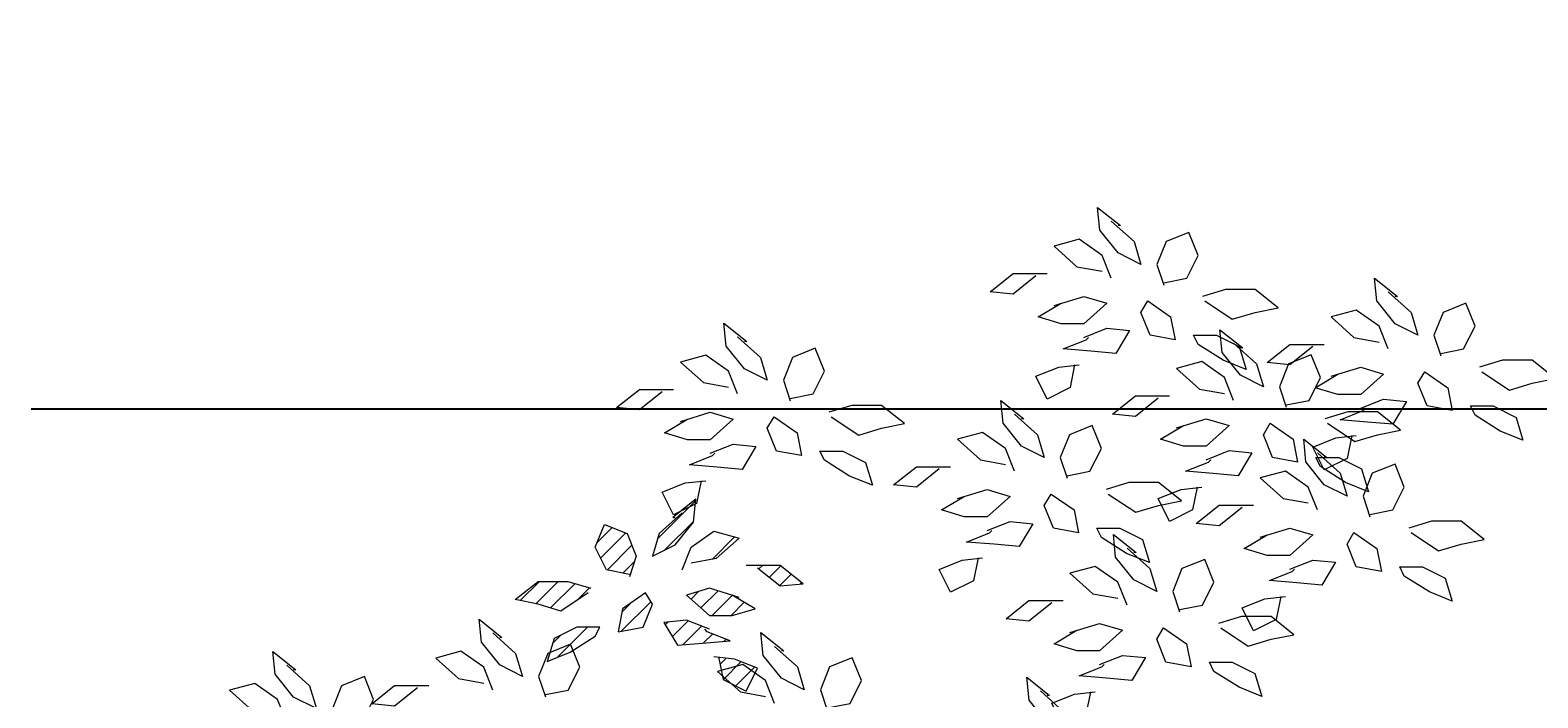
# Model space of a CAD drawing. Units: inches. Extents: x 1770 to 2988, y 1161 to 3221.
# Tile 42 of 44: x 2655 to 2745, y 2825 to 2865. Entities that reach past the tile are written whole.
import ezdxf

# ---------------------------------------------------------------- set-up
doc = ezdxf.new("R2010")
doc.units = ezdxf.units.IN
doc.layers.add('A-ANNO-DIMS', color=2, linetype='Continuous', lineweight=18)
doc.layers.add('trees1', color=250, linetype='Continuous', lineweight=13)
doc.styles.get("Standard").update_dxf_attribs({"font": 'arial.ttf'})
doc.dimstyles.get("Standard").update_dxf_attribs({"dimtxt": 0.18, "dimasz": 0.18, "dimexe": 0.18, "dimexo": 0.0625, "dimgap": 0.09, "dimtad": 0, "dimtih": 1, "dimtoh": 1, "dimdec": 4, "dimzin": 0, "dimdsep": 46, "dimtxsty": 'Standard', "dimcen": 0.09, "dimadec": 0, "dimazin": 0, "dimtfac": 1, "dimtdec": 4, "dimtofl": 0, "dimtmove": 0, "dimatfit": 3, "dimfxl": 1, "dimtolj": 1, "dimtzin": 0, "dimarcsym": 0})

# ---------------------------------------------------------------- blocks, each defined once
blk = doc.blocks.new('*X8')
at = {"color": 0}
for p, q in [((0.637, -0.8479), (0.6441, -0.8408)), ((0.6463, -0.8563), (0.6624, -0.8402)), ((0.6568, -0.8635), (0.676, -0.8443)), ((0.6745, -0.8635), (0.687, -0.8509))]:
    blk.add_line(p, q, dxfattribs=at)
blk = doc.blocks.new('*X14')
at = {"color": 0}
blk.add_line((0.6567, -0.8106), (0.6779, -0.7894), dxfattribs=at)
blk = doc.blocks.new('*X9')
at = {"color": 0}
for p, q in [((0.7007, -0.8195), (0.704, -0.8163)), ((0.7106, -0.8274), (0.7213, -0.8167)), ((0.7204, -0.8352), (0.7311, -0.8245)), ((0.7396, -0.8337), (0.7409, -0.8324))]:
    blk.add_line(p, q, dxfattribs=at)
blk = doc.blocks.new('*X7')
at = {"color": 0}
for p, q in [((0.6642, -0.9091), (0.6699, -0.9034)), ((0.6673, -0.9237), (0.6842, -0.9068)), ((0.6791, -0.9296), (0.6968, -0.9118))]:
    blk.add_line(p, q, dxfattribs=at)
blk = doc.blocks.new('*X11')
at = {"color": 0}
for p, q in [((0.5716, -0.8779), (0.5992, -0.8504)), ((0.5721, -0.8598), (0.5799, -0.852))]:
    blk.add_line(p, q, dxfattribs=at)
blk = doc.blocks.new('*X12')
at = {"color": 0}
for p, q in [((0.4764, -0.8494), (0.4945, -0.8313)), ((0.4911, -0.8524), (0.5122, -0.8313)), ((0.5049, -0.8563), (0.5279, -0.8333)), ((0.5296, -0.8493), (0.5415, -0.8374))]:
    blk.add_line(p, q, dxfattribs=at)
blk = doc.blocks.new('*X10')
at = {"color": 0}
for p, q in [((0.5118, -0.9024), (0.54, -0.8742)), ((0.5068, -0.8897), (0.5149, -0.8816))]:
    blk.add_line(p, q, dxfattribs=at)
blk = doc.blocks.new('*X6')
at = {"color": 0}
for p, q in [((0.6127, -0.8722), (0.6154, -0.8695)), ((0.6193, -0.8833), (0.6342, -0.8684)), ((0.6293, -0.8909), (0.6469, -0.8734)), ((0.6488, -0.8892), (0.6573, -0.8806)), ((0.6681, -0.8876), (0.67, -0.8857))]:
    blk.add_line(p, q, dxfattribs=at)
blk = doc.blocks.new('*X13')
at = {"color": 0}
for p, q in [((0.5486, -0.7949), (0.5629, -0.7806)), ((0.552, -0.8092), (0.5755, -0.7857)), ((0.5582, -0.8207), (0.5814, -0.7974)), ((0.5729, -0.8236), (0.5839, -0.8126))]:
    blk.add_line(p, q, dxfattribs=at)
blk = doc.blocks.new('*X15')
at = {"color": 0}
for p, q in [((0.6056, -0.7909), (0.6413, -0.7553)), ((0.6124, -0.8018), (0.6393, -0.7749))]:
    blk.add_line(p, q, dxfattribs=at)
blk = doc.blocks.new('tree342')
at = {"color": 0}
for points in [[(4.4, 2257.6), (25.9, 2238.3), (32.3, 2216.8), (10.8, 2227.6), (-6.3, 2249), (-8.5, 2270.5), (13, 2253.3), (10.8, 2253.3)], [(4.4, 2204), (-4.2, 2225.4), (-25.7, 2240.5), (-49.3, 2234), (-27.8, 2214.7), (-4.2, 2210.4)], [(53.8, 2199.7), (75.3, 2204), (86, 2225.4), (77.4, 2246.9), (55.9, 2238.3), (47.3, 2216.8), (53.8, 2197.5)], [(-66.5, 2206.1), (-87.9, 2188.9), (-109.4, 2191.1), (-87.9, 2208.3), (-55.7, 2208.3)], [(264.7, 2191.1), (286.2, 2171.8), (292.7, 2150.3), (271.2, 2161), (254, 2182.5), (251.9, 2203.9), (273.3, 2186.8), (271.2, 2186.8)], [(-49.3, 2178.2), (-21.4, 2186.8), (0.1, 2180.4), (-21.4, 2161), (-42.8, 2161), (-64.3, 2167.5), (-42.8, 2180.4)], [(92.4, 2182.5), (118.2, 2165.3), (139.7, 2171.8), (161.2, 2176.1), (139.7, 2193.2), (111.8, 2193.2), (90.3, 2186.8)], [(264.7, 2137.4), (256.2, 2158.9), (234.7, 2173.9), (211.1, 2167.5), (232.5, 2148.1), (256.2, 2143.9)], [(314.1, 2133.1), (335.6, 2137.4), (346.3, 2158.9), (337.8, 2180.3), (316.3, 2171.8), (307.7, 2150.3), (314.1, 2131)], [(-346.8, 2148.7), (-325.3, 2129.4), (-318.9, 2107.9), (-340.3, 2118.7), (-357.5, 2140.1), (-359.7, 2161.6), (-338.2, 2144.4), (-340.3, 2144.4)], [(-21.4, 2148.2), (0.1, 2156.8), (21.6, 2154.6), (8.7, 2133.2), (-14.9, 2135.3), (-40.7, 2137.4), (-19.2, 2146), (-17.1, 2148.2)], [(119.4, 2142.7), (140.9, 2123.3), (147.4, 2101.9), (125.9, 2112.6), (108.7, 2134.1), (106.5, 2155.5), (128, 2138.4), (125.9, 2138.4)], [(193.9, 2139.6), (172.4, 2122.4), (150.9, 2124.5), (172.4, 2141.7), (204.6, 2141.7)], [(-346.8, 2095.1), (-355.4, 2116.5), (-376.8, 2131.5), (-400.5, 2125.1), (-379, 2105.8), (-355.4, 2101.5)], [(-297.4, 2090.8), (-275.9, 2095.1), (-265.2, 2116.5), (-273.8, 2138), (-295.2, 2129.4), (-303.8, 2107.9), (-297.4, 2088.6)], [(168.8, 2084.7), (190.3, 2089), (201, 2110.5), (192.4, 2131.9), (171, 2123.3), (162.4, 2101.9), (168.8, 2082.6)], [(352.8, 2116), (378.6, 2098.8), (400, 2105.2), (421.5, 2109.5), (400, 2126.7), (372.1, 2126.7), (350.6, 2120.2)], [(-30, 2122.4), (-34.3, 2101), (-55.7, 2090.2), (-66.5, 2111.7), (-45, 2120.3), (-25.7, 2122.4)], [(119.4, 2089), (110.8, 2110.5), (89.4, 2125.5), (65.7, 2119.1), (87.2, 2099.7), (110.8, 2095.4)], [(211.1, 2111.7), (239, 2120.2), (260.4, 2113.8), (239, 2094.5), (217.5, 2094.5), (196, 2100.9), (217.5, 2113.8)], [(-417.6, 2097.2), (-439.1, 2080), (-460.6, 2082.2), (-439.1, 2099.4), (-406.9, 2099.4)], [(-258.7, 2073.6), (-233, 2056.4), (-211.5, 2062.9), (-190, 2067.2), (-211.5, 2084.3), (-239.4, 2084.3), (-260.9, 2077.9)], [(-86.4, 2076.1), (-64.9, 2056.8), (-58.5, 2035.3), (-80, 2046.1), (-97.2, 2067.5), (-99.3, 2089), (-77.8, 2071.8), (-80, 2071.8)], [(48.6, 2091.2), (27.1, 2074), (5.6, 2076.1), (27.1, 2093.3), (59.3, 2093.3)], [(239, 2081.6), (260.4, 2090.2), (281.9, 2088.1), (269, 2066.6), (245.4, 2068.7), (219.6, 2070.9), (241.1, 2079.5), (243.3, 2081.6)], [(-400.5, 2069.3), (-372.5, 2077.9), (-351.1, 2071.5), (-372.5, 2052.1), (-394, 2052.1), (-415.5, 2058.6), (-394, 2071.5)], [(65.7, 2063.3), (93.7, 2071.8), (115.1, 2065.4), (93.7, 2046.1), (72.2, 2046.1), (50.7, 2052.5), (72.2, 2065.4)], [(207.5, 2067.6), (233.2, 2050.4), (254.7, 2056.8), (276.2, 2061.1), (254.7, 2078.3), (226.8, 2078.3), (205.3, 2071.8)], [(-86.4, 2022.5), (-95, 2043.9), (-116.5, 2058.9), (-140.1, 2052.5), (-118.6, 2033.2), (-95, 2028.9)], [(-37, 2018.2), (-15.6, 2022.5), (-4.8, 2043.9), (-13.4, 2065.4), (-34.9, 2056.8), (-43.5, 2035.3), (-37, 2016)], [(230.4, 2055.9), (226.1, 2034.4), (204.6, 2023.7), (193.9, 2045.1), (215.4, 2053.7), (234.7, 2055.9)], [(-372.5, 2039.3), (-351.1, 2047.8), (-329.6, 2045.7), (-342.5, 2024.2), (-366.1, 2026.4), (-391.9, 2028.5), (-370.4, 2037.1), (-368.2, 2039.3)], [(93.7, 2033.2), (115.1, 2041.8), (136.6, 2039.7), (123.7, 2018.2), (100.1, 2020.3), (74.3, 2022.5), (95.8, 2031.1), (98, 2033.2)], [(198.1, 2039.8), (219.6, 2020.5), (226.1, 1999), (204.6, 2009.8), (187.4, 2031.2), (185.3, 2052.7), (206.7, 2035.5), (204.6, 2035.5)], [(-157.3, 2024.6), (-178.8, 2007.4), (-200.2, 2009.6), (-178.8, 2026.7), (-146.6, 2026.7)], [(247.5, 1981.9), (269, 1986.2), (279.7, 2007.6), (271.2, 2029.1), (249.7, 2020.5), (241.1, 1999), (247.5, 1979.7)], [(-381.1, 2013.5), (-385.4, 1992.1), (-406.9, 1981.3), (-417.6, 2002.8), (-396.2, 2011.4), (-376.8, 2013.5)], [(198.1, 1986.2), (189.6, 2007.6), (168.1, 2022.6), (144.5, 2016.2), (165.9, 1996.9), (189.6, 1992.6)], [(-140.1, 1996.7), (-112.2, 2005.3), (-90.7, 1998.8), (-112.2, 1979.5), (-133.7, 1979.5), (-155.1, 1986), (-133.7, 1998.8)], [(1.6, 2001), (27.4, 1983.8), (48.9, 1990.3), (70.3, 1994.6), (48.9, 2011.7), (21, 2011.7), (-0.5, 2005.3)], [(85.1, 2007.5), (80.8, 1986), (59.3, 1975.3), (48.6, 1996.7), (70, 2005.3), (89.4, 2007.5)], [(-399, 1983.2), (-420.5, 1963.9), (-426.9, 1942.5), (-405.5, 1953.2), (-388.3, 1974.6), (-386.1, 1996.1), (-407.6, 1978.9), (-405.5, 1978.9)], [(127.3, 1988.3), (105.8, 1971.1), (84.3, 1973.3), (105.8, 1990.4), (138, 1990.4)], [(-448.4, 1925.3), (-469.9, 1929.6), (-480.6, 1951), (-472, 1972.5), (-450.6, 1963.9), (-442, 1942.5), (-448.4, 1923.1)], [(-112.2, 1966.7), (-90.7, 1975.2), (-69.2, 1973.1), (-82.1, 1951.6), (-105.7, 1953.8), (-131.5, 1955.9), (-110, 1964.5), (-107.9, 1966.7)], [(286.2, 1964.7), (312, 1947.5), (333.4, 1954), (354.9, 1958.3), (333.4, 1975.4), (305.5, 1975.4), (284, 1969)], [(-399, 1929.6), (-390.4, 1951), (-369, 1966.1), (-345.3, 1959.6), (-366.8, 1940.3), (-390.4, 1936)], [(19.3, 1950.2), (40.8, 1930.9), (47.2, 1909.4), (25.7, 1920.2), (8.5, 1941.6), (6.4, 1963.1), (27.9, 1945.9), (25.7, 1945.9)], [(144.5, 1960.4), (172.4, 1969), (193.8, 1962.5), (172.4, 1943.2), (150.9, 1943.2), (129.4, 1949.7), (150.9, 1962.5)], [(-328.2, 1931.7), (-306.7, 1914.6), (-285.2, 1916.7), (-306.7, 1933.9), (-338.9, 1933.9)], [(-120.8, 1940.9), (-125.1, 1919.4), (-146.6, 1908.7), (-157.3, 1930.2), (-135.8, 1938.8), (-116.5, 1940.9)], [(19.3, 1896.5), (10.7, 1918), (-10.8, 1933), (-34.4, 1926.6), (-12.9, 1907.3), (10.7, 1903)], [(68.7, 1892.3), (90.2, 1896.5), (100.9, 1918), (92.3, 1939.5), (70.8, 1930.9), (62.2, 1909.4), (68.7, 1890.1)], [(172.4, 1930.4), (193.8, 1938.9), (215.3, 1936.8), (202.4, 1915.3), (178.8, 1917.5), (153, 1919.6), (174.5, 1928.2), (176.7, 1930.4)], [(-487.1, 1908.1), (-512.8, 1891), (-534.3, 1897.4), (-555.8, 1901.7), (-534.3, 1918.9), (-506.4, 1918.9), (-484.9, 1912.4)], [(-345.3, 1903.8), (-373.3, 1912.4), (-394.7, 1906), (-373.3, 1886.7), (-351.8, 1886.7), (-330.3, 1893.1), (-351.8, 1906)], [(-51.6, 1898.7), (-73.1, 1881.5), (-94.5, 1883.7), (-73.1, 1900.8), (-40.8, 1900.8)], [(163.8, 1904.6), (159.5, 1883.1), (138, 1872.4), (127.3, 1893.9), (148.8, 1902.5), (168.1, 1904.6)], [(107.3, 1875.1), (133.1, 1857.9), (154.6, 1864.4), (176, 1868.6), (154.6, 1885.8), (126.7, 1885.8), (105.2, 1879.4)], [(-576.8, 1870.4), (-555.4, 1851.1), (-548.9, 1829.6), (-570.4, 1840.3), (-587.6, 1861.8), (-589.7, 1883.3), (-568.3, 1866.1), (-570.4, 1866.1)], [(-373.3, 1873.8), (-394.7, 1882.4), (-416.2, 1880.2), (-403.3, 1858.8), (-379.7, 1860.9), (-353.9, 1863.1), (-375.4, 1871.6), (-377.5, 1873.8)], [(-312, 1857.8), (-290.5, 1838.5), (-284.1, 1817), (-305.5, 1827.8), (-322.7, 1849.2), (-324.9, 1870.7), (-303.4, 1853.5), (-305.5, 1853.5)], [(-34.4, 1870.8), (-6.5, 1879.4), (15, 1872.9), (-6.5, 1853.6), (-28, 1853.6), (-49.4, 1860.1), (-28, 1872.9)], [(-527.5, 1812.4), (-506, 1816.7), (-495.2, 1838.2), (-503.8, 1859.7), (-525.3, 1851.1), (-533.9, 1829.6), (-527.5, 1810.3)], [(-770.6, 1840.1), (-749.1, 1820.8), (-742.7, 1799.4), (-764.1, 1810.1), (-781.3, 1831.6), (-783.5, 1853), (-762, 1835.8), (-764.1, 1835.8)], [(-576.8, 1816.7), (-585.4, 1838.2), (-606.9, 1853.2), (-630.5, 1846.8), (-609.1, 1827.5), (-585.4, 1823.2)], [(-364.7, 1848), (-360.4, 1826.6), (-338.9, 1815.8), (-328.2, 1837.3), (-349.6, 1845.9), (-369, 1848)], [(-262.6, 1799.9), (-241.1, 1804.2), (-230.4, 1825.6), (-239, 1847.1), (-260.4, 1838.5), (-269, 1817), (-262.6, 1797.7)], [(-6.5, 1840.8), (15, 1849.3), (36.5, 1847.2), (23.6, 1825.7), (0, 1827.9), (-25.8, 1830), (-4.3, 1838.6), (-2.2, 1840.8)], [(-721.2, 1782.2), (-699.7, 1786.5), (-689, 1807.9), (-697.6, 1829.4), (-719.1, 1820.8), (-727.6, 1799.4), (-721.2, 1780)], [(-312, 1804.2), (-320.6, 1825.6), (-342, 1840.6), (-365.7, 1834.2), (-344.2, 1814.9), (-320.6, 1810.6)], [(-62.2, 1815.9), (-40.7, 1796.6), (-34.3, 1775.2), (-55.8, 1785.9), (-72.9, 1807.3), (-75.1, 1828.8), (-53.6, 1811.6), (-55.8, 1811.6)], [(-770.6, 1786.5), (-779.2, 1807.9), (-800.7, 1823), (-824.3, 1816.5), (-802.8, 1797.2), (-779.2, 1792.9)], [(-647.7, 1818.9), (-669.2, 1801.7), (-690.7, 1803.9), (-669.2, 1821), (-637, 1821)], [(-15.1, 1815), (-19.4, 1793.5), (-40.8, 1782.8), (-51.6, 1804.3), (-30.1, 1812.9), (-10.8, 1815)]]:
    blk.add_lwpolyline(points, dxfattribs=at)
for points in [[(60.2, 2167.5), (64.5, 2146), (40.9, 2150.3), (32.3, 2171.8), (38.8, 2182.5)], [(103.2, 2150.3), (124.7, 2139.6), (131.1, 2118.1), (109.6, 2126.7), (86, 2141.7), (81.7, 2150.3)], [(320.6, 2100.9), (324.9, 2079.5), (301.3, 2083.8), (292.7, 2105.2), (299.1, 2116)], [(363.5, 2083.8), (385, 2073), (391.4, 2051.6), (370, 2060.2), (346.3, 2075.2), (342.1, 2083.8)], [(-290.9, 2058.6), (-286.6, 2037.1), (-310.3, 2041.4), (-318.9, 2062.9), (-312.4, 2073.6)], [(175.3, 2052.5), (179.6, 2031.1), (155.9, 2035.4), (147.4, 2056.8), (153.8, 2067.6)], [(-248, 2041.4), (-226.5, 2030.7), (-220.1, 2009.2), (-241.5, 2017.8), (-265.2, 2032.8), (-269.5, 2041.4)], [(218.2, 2035.4), (239.7, 2024.6), (246.1, 2003.2), (224.7, 2011.8), (201, 2026.8), (196.7, 2035.4)], [(-30.6, 1986), (-26.3, 1964.5), (-49.9, 1968.8), (-58.5, 1990.3), (-52.1, 2001)], [(12.4, 1968.8), (33.8, 1958.1), (40.3, 1936.6), (18.8, 1945.2), (-4.8, 1960.2), (-9.1, 1968.8)], [(254, 1949.7), (258.3, 1928.2), (234.6, 1932.5), (226.1, 1954), (232.5, 1964.7)], [(296.9, 1932.5), (318.4, 1921.8), (324.8, 1900.3), (303.4, 1908.9), (279.7, 1923.9), (275.5, 1932.5)], [(-454.9, 1893.1), (-459.2, 1871.6), (-435.5, 1875.9), (-426.9, 1897.4), (-433.4, 1908.1)], [(-497.8, 1875.9), (-519.3, 1865.2), (-525.7, 1843.7), (-504.2, 1852.3), (-480.6, 1867.3), (-476.3, 1875.9)], [(75.1, 1860.1), (79.4, 1838.6), (55.8, 1842.9), (47.2, 1864.4), (53.6, 1875.1)], [(118.1, 1842.9), (139.5, 1832.2), (146, 1810.7), (124.5, 1819.3), (100.9, 1834.3), (96.6, 1842.9)]]:
    blk.add_lwpolyline(points, close=True, dxfattribs=at)
at = {"color": 0, "xscale": 1000, "yscale": 1000, "zscale": 1000}
for name in ['*X15', '*X13', '*X14', '*X9', '*X12', '*X11', '*X8', '*X10', '*X6', '*X7']:
    blk.add_blockref(name, (-1027.5, 2750.2), dxfattribs=at)
blk = doc.blocks.new('*D98')
at = {"layer": 'A-ANNO-DIMS', "color": 0, "lineweight": -2, "transparency": 16777216}
for p, q in [((2655.505, 2842.297), (2801.915, 2842.297)), ((2801.735, 2842.117), (2801.735, 2824.479)), ((2801.735, 2806.477), (2801.735, 2824.115)), ((2620.113, 2806.297), (2801.915, 2806.297))]:
    blk.add_line(p, q, dxfattribs=at)
at = {"layer": 'A-ANNO-DIMS', "color": 0, "transparency": 16777216}
for points in [[(2801.705, 2842.117), (2801.765, 2842.117), (2801.735, 2842.297)], [(2801.705, 2806.477), (2801.765, 2806.477), (2801.735, 2806.297)]]:
    blk.add_solid(points, dxfattribs=at)
at = {"layer": 'Defpoints', "color": 0, "transparency": 16777216}
for p in [(2655.443, 2842.297), (2801.735, 2842.297), (2620.051, 2806.297)]:
    blk.add_point(p, dxfattribs=at)
at = {"layer": 'A-ANNO-DIMS', "color": 0, "transparency": 16777216, "insert": (2801.735, 2824.297), "char_height": 0.18, "attachment_point": 5}
blk.add_mtext('\\A1;36', dxfattribs=at)
blk = doc.blocks.new('*D99')
at = {"layer": 'A-ANNO-DIMS', "color": 0, "lineweight": -2, "transparency": 16777216}
for p, q in [((2655.505, 2871.794), (2801.915, 2871.794)), ((2801.735, 2871.614), (2801.735, 2857.228)), ((2801.735, 2842.477), (2801.735, 2856.864)), ((2655.505, 2842.297), (2801.915, 2842.297))]:
    blk.add_line(p, q, dxfattribs=at)
at = {"layer": 'A-ANNO-DIMS', "color": 0, "transparency": 16777216}
for points in [[(2801.705, 2871.614), (2801.765, 2871.614), (2801.735, 2871.794)], [(2801.705, 2842.477), (2801.765, 2842.477), (2801.735, 2842.297)]]:
    blk.add_solid(points, dxfattribs=at)
at = {"layer": 'Defpoints', "color": 0, "transparency": 16777216}
for p in [(2655.443, 2871.794), (2801.735, 2871.794), (2655.443, 2842.297)]:
    blk.add_point(p, dxfattribs=at)
at = {"layer": 'A-ANNO-DIMS', "color": 0, "transparency": 16777216, "insert": (2801.735, 2857.046), "char_height": 0.18, "attachment_point": 5}
blk.add_mtext('\\A1;29.5', dxfattribs=at)

msp = doc.modelspace()

# ---------------------------------------------------------------- block references
at = {"layer": 'trees1', "xscale": 0.063143750371755, "yscale": 0.063143750371755, "zscale": 0.063143750371755}
msp.add_blockref('tree342', (2719.3275, 2710.8976), dxfattribs=at)

# ---------------------------------------------------------------- dimensions: what is measured, and where the dimension line sits
at = {"layer": 'A-ANNO-DIMS'}
for base, p1, p2, override, picture, middle in [((2801.7346, 2871.7944), (2655.443, 2842.2969), (2655.443, 2871.7944), {"dimdec": 1, "dimlfac": 1, "dimrnd": 0, "dimzin": 0, "dimdsep": 46, "dimlunit": 2}, '*D99', (2801.7346, 2857.0456)), ((2801.7346, 2842.2969), (2620.0508, 2806.2969), (2655.443, 2842.2969), {"dimdec": 0, "dimlfac": 1, "dimrnd": 0, "dimzin": 0, "dimdsep": 46, "dimlunit": 2}, '*D98', (2801.7346, 2824.2969))]:
    dim = msp.add_linear_dim(base=base, p1=p1, p2=p2, angle=90, dimstyle='Standard', override=override, dxfattribs=at)
    dim.commit()
    dim.dimension.update_dxf_attribs({"geometry": picture, "text_midpoint": middle})

doc.saveas('drawing.dxf')
